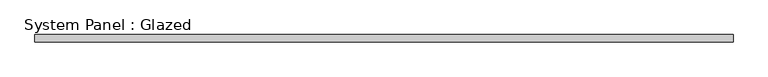
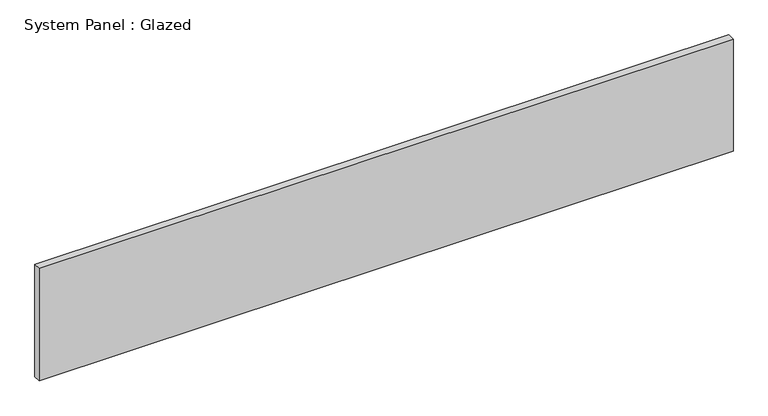
"""IFC4 building model written with IfcOpenShell, lengths in millimetres: plate geometry, System Panel : Glazed."""

from ifc_helpers import new_model, si_unit, origin, origin_with_axes, place, context, project, spatial, polyline, outline, extrude, source, transform, mapped, element, save


def system_panel_glazed_07248474(model_context):
    return source(origin(), model_context, "Body", "SweptSolid", [
        extrude(outline(polyline([(1222.375, 19.05), (-1222.375, 19.05), (-1222.375, 44.45), (1222.375, 44.45), (1222.375, 19.05)])), origin_with_axes(), (0.0, 0.0, 1.0), 418.3568067),
    ])


if __name__ == "__main__":
    model = new_model("IFC4")
    model_context = context("Model", 3, world=origin())
    ifc_project = project(units=[si_unit("LENGTHUNIT", "METRE", prefix="MILLI")], contexts=[model_context])
    site = spatial("IfcSite", under=ifc_project)
    building = spatial("IfcBuilding", under=site)
    placement = place(None, origin())
    system_panel_glazed_shape = system_panel_glazed_07248474(model_context)
    element("IfcPlate", 1, ObjectType="System Panel : Glazed", at=placement, inside=building, context=model_context, shape_type="MappedRepresentation", body=[
        mapped(system_panel_glazed_shape, transform((0.0, 0.0, 0.0), x_axis=(1.0, 0.0, 0.0), y_axis=(0.0, 1.0, 0.0), z_axis=(0.0, 0.0, 1.0))),
    ])
    save(model, "model.ifc")

# Revit data of these elements
# Type "System Panel : Glazed"
#   Construction Type Id = "GSP4R"
#   Analytic Construction = "1/8 in Pilkington single glazing"
#   Visual Light Transmittance = 0.9
#   Solar Heat Gain Coefficient = 0.86
#   Heat Transfer Coefficient (U) = 1.18115 BTU/(h·ft²·°F)
#   Define Thermal Properties by = 1
# Element 1 (IfcPlate, "System Panel : Glazed")
#   Materials on its faces: "Glass"
# Materials
#   "Glass": class "Glass", colour RGB 0 128 192, transparency 0.75, Description = "Soda Lime Glass", Cost = 0
